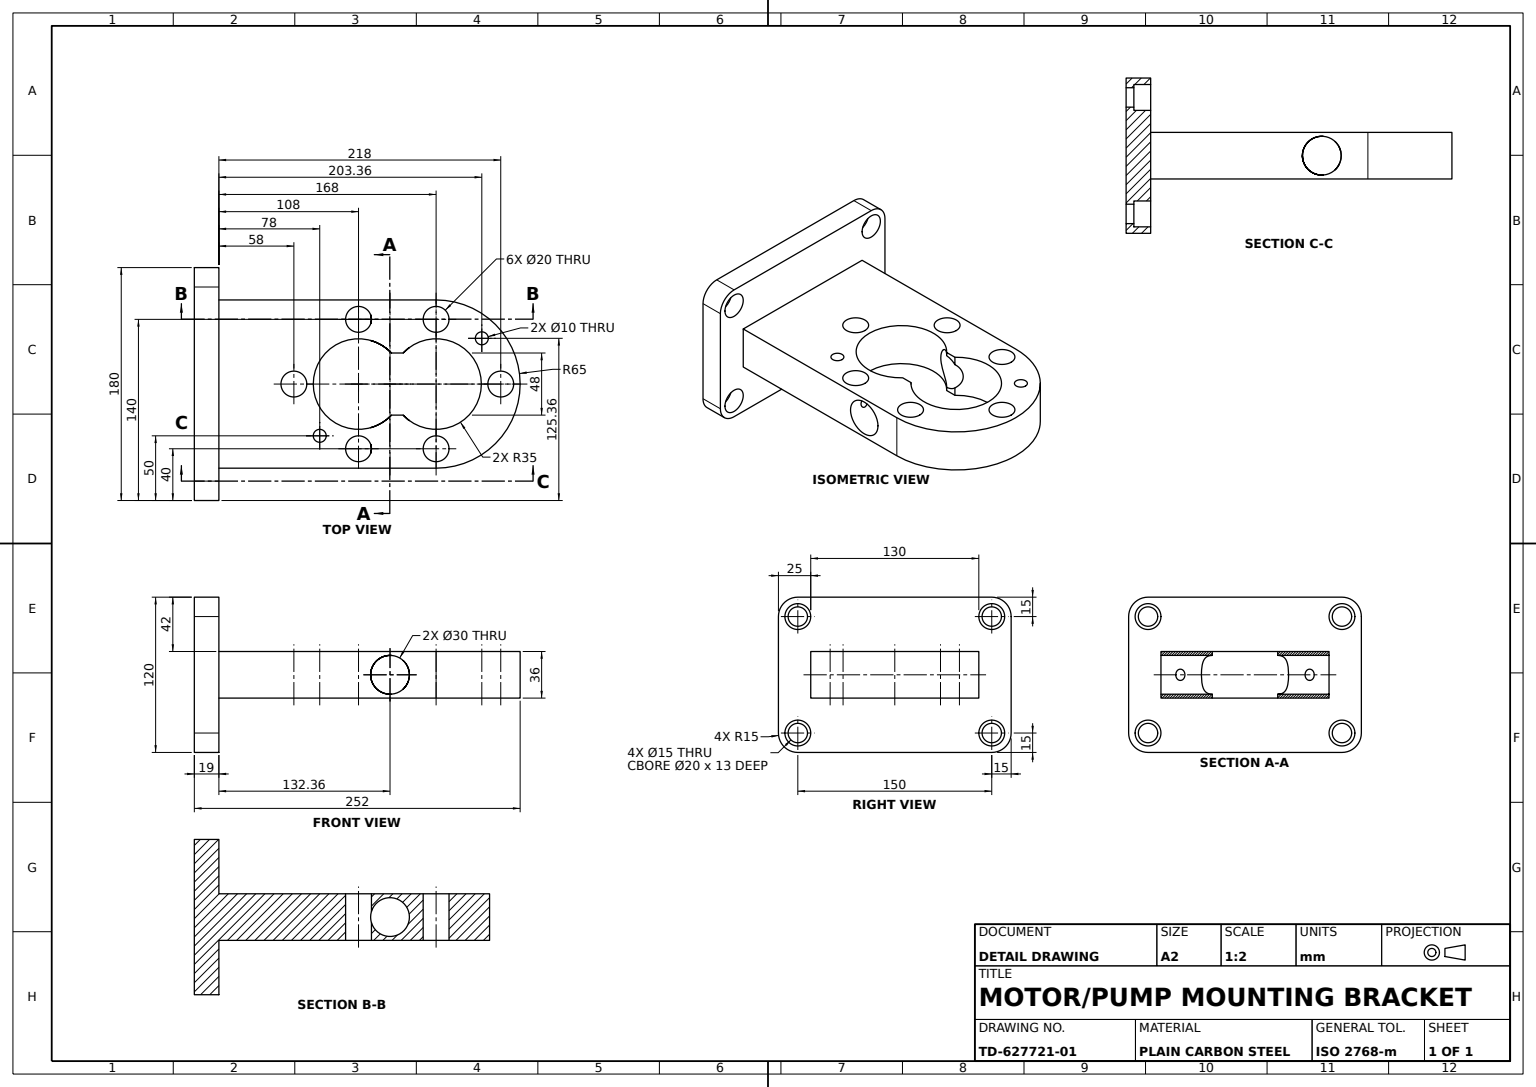
SolidWorks part; units mm, degrees
material "Plain Carbon Steel"
ref_plane "Front Plane" through (0, 0, 0) normal (0, 0, 1) x (1, 0, 0)
ref_plane "Top Plane" through (0, 0, 0) normal (0, 1, 0) x (1, 0, 0)
ref_plane "Right Plane" through (0, 0, 0) normal (1, 0, 0) x (0, 0, -1)
sketch "Flange Profile Sketch" plane through (0, 0, 0) normal (0, 0, 1) x (1, 0, 0)
  line L0 (0, 0) -> (180, 0)
  line L1 (180, 0) -> (180, 120)
  line L2 (180, 120) -> (0, 120)
  line L3 (0, 120) -> (0, 0)
  dimension "D1" = 180
  dimension "D2" = 120
extrude "Mounting Flange" add sketch "Flange Profile Sketch" along normal blind 19
ref_plane "Plane1" through (0, 60, 0) normal (0, 1, 0) x (1, 0, 0)
sketch "Support Arm Profile Sketch" plane through (0, 60, 0) normal (0, 1, 0) x (1, 0, 0)
  line L0 (180, 0) -> (0, 0) construction
  line L1 (25, 168) -> (25, 0)
  line L2 (155, 168) -> (155, 0)
  line L3 (155, 0) -> (25, 0)
  arc A0 (155, 168) -> (25, 168) centre (90, 168) ccw
  dimension "D1" = 130
  dimension "D2" = 168
  dimension "D3" = 25
extrude "Support Arm" add sketch "Support Arm Profile Sketch" along normal mid plane 36
sketch "Bearing Bore and Bolt Holes Sketch" plane through (0, 78, 0) normal (0, 1, 0) x (1, 0, 0)
  line L0 (90, 168) -> (90, 218) construction
  line L1 (90, 168) -> (90, 118) construction
  line L2 (90, 168) -> (40, 168) construction
  line L3 (90, 168) -> (140, 168) construction
  line L4 (90, 168) -> (90, 108) construction
  line L5 (66, 142.5245) -> (66, 133.4755)
  line L6 (114, 142.5245) -> (114, 133.4755)
  line L7 (90, 73) -> (90, 58) construction
  line L10 (90, 108) -> (90, 73) construction
  line L13 (90, 118) -> (40, 168) construction
  line L14 (90, 118) -> (40, 118) construction
  line L15 (90, 118) -> (130, 78) construction
  line L16 (90, 168) -> (54.6447, 203.3553) construction
  arc A0 (114, 142.5245) -> (66, 142.5245) centre (90, 168) ccw
  circle A2 centre (90, 218) radius 10
  circle A3 centre (140, 168) radius 10
  circle A5 centre (40, 168) radius 10
  circle A6 centre (90, 118) radius 10 [skipped]
  arc A7 (66, 133.4755) -> (114, 133.4755) centre (90, 108) ccw
  arc A18 (50, 138) -> (130, 138) centre (90, 108) ccw construction
  arc A19 (130, 138) -> (50, 138) centre (90, 168) ccw construction
  circle A20 centre (90, 58) radius 10
  circle A21 centre (40, 108) radius 10
  circle A23 centre (140, 108) radius 10
  circle A24 centre (90, 158) radius 10 [skipped]
  circle A25 centre (54.6447, 203.3553) radius 5
  circle A26 centre (130, 78) radius 5
  dimension "D1" = 70
  dimension "D2" = 100
  dimension "D3" = 20
  dimension "D7" = 70
  dimension "D9" = 100
  dimension "D11" = 218
  dimension "D15" = 20
  dimension "D16" = 4
  dimension "D18" = 108
  dimension "D19" = 45
  dimension "D20" = 10
  dimension "D22" = 10
  dimension "D5" = 140
  dimension "D6" = 40
  dimension "D8" = 108
  dimension "D12" = 73
  dimension "D13" = 9.049
  dimension "D14" = 9.049
  dimension "D17" = 40
  dimension "D10" = 118
  dimension "D21" = 45
  dimension "D4" = 4
extrude "Bearing Bore and Bolt Holes" cut sketch "Bearing Bore and Bolt Holes Sketch" against normal blind 36
sketch "Cross Hole Sketch" plane through (25, 0, 0) normal (-1, 0, 0) x (0, 0, 1)
  line L0 (-168, 42) -> (0, 42) construction
  circle A0 centre (-132.3577, 60) radius 15
  dimension "D1" = 30
  dimension "D2" = 132.3577
  dimension "D3" = 18
extrude "Cross Hole Ø30" cut sketch "Cross Hole Sketch" against normal through all
fillet "Flange Corner Fillets R15" radius 15 4 edges at (0, 120, 9.5) (0, 0, 9.5) (180, 0, 9.5) (180, 120, 9.5)
sketch "Flange Mounting Holes Sketch" plane through (0, 0, 0) normal (0, 0, -1) x (-1, 0, 0)
  circle A0 centre (-165, 15) radius 7.5
  circle A1 centre (-15, 15) radius 7.5
  circle A2 centre (-15, 105) radius 7.5
  circle A3 centre (-165, 105) radius 7.5
  dimension "D1" = 15
  dimension "D2" = 15
  dimension "D3" = 15
  dimension "D4" = 15
extrude "Flange Mounting Holes" cut sketch "Flange Mounting Holes Sketch" against normal blind 36
sketch "Flange Secondary Cut Sketch" plane through (0, 0, 0) normal (0, 0, -1) x (-1, 0, 0)
  circle A0 centre (-165, 105) radius 10
  circle A1 centre (-15, 105) radius 10
  circle A2 centre (-15, 15) radius 10
  circle A3 centre (-165, 15) radius 10
  dimension "D1" = 20
  dimension "D2" = 20
  dimension "D3" = 20
  dimension "D4" = 20
extrude "Flange Secondary Cut" cut sketch "Flange Secondary Cut Sketch" against normal blind 13
